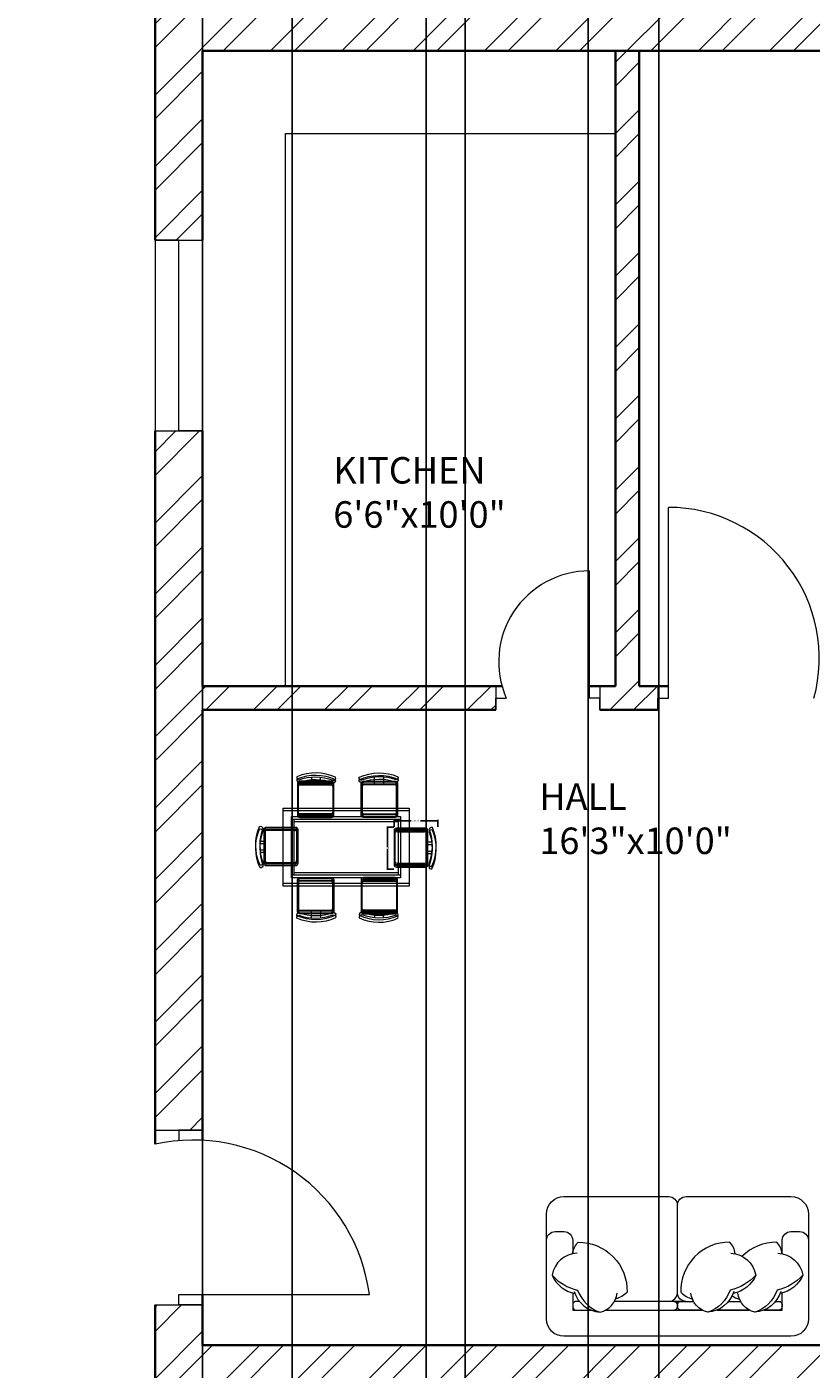
# Model space of a CAD drawing. Units: inches. Extents: x 2552 to 3217, y 1417 to 2737.
# Tile 5 of 25: x 2885 to 3033, y 1631 to 1885. Entities that reach past the tile are written whole.
import ezdxf

# ---------------------------------------------------------------- set-up
doc = ezdxf.new("R2010")
doc.units = ezdxf.units.IN
for name, color, linetype, lineweight in [('A-ANNO-DIMS', 2, 'Continuous', 18), ('A-AREA-IDEN', 7, 'Continuous', 18), ('A-DOOR', 21, 'Continuous', 18), ('A-FLOR-CASE', 9, 'Continuous', 18), ('A-FURN', 8, 'Continuous', 13), ('A-GLAZ', 161, 'Continuous', 18), ('A-WALL', 7, 'Continuous', 35), ('A-WALL-PATT', 217, 'Continuous', 13)]:
    doc.layers.add(name, color=color, linetype=linetype, lineweight=lineweight)
doc.styles.get("Standard").update_dxf_attribs({"font": 'arial.ttf'})
doc.dimstyles.get("Standard").update_dxf_attribs({"dimtxt": 0.18, "dimasz": 0.18, "dimexe": 0.18, "dimexo": 0.0625, "dimgap": 0.09, "dimtad": 0, "dimtih": 1, "dimtoh": 1, "dimdec": 4, "dimzin": 0, "dimdsep": 46, "dimtxsty": 'Standard', "dimcen": 0.09, "dimadec": 0, "dimazin": 0, "dimtfac": 1, "dimtdec": 4, "dimtofl": 0, "dimtmove": 0, "dimatfit": 3, "dimfxl": 1, "dimtolj": 1, "dimtzin": 0, "dimarcsym": 0})

# ---------------------------------------------------------------- blocks, each defined once
blk = doc.blocks.new('TABLE-DINING-RECT')
for points in [[(0, 14.74), (23.77, 14.74), (23.77, 0.48), (0, 0.48)], [(0, 14.74), (23.77, 14.74), (23.77, 0.48), (0, 0.48)], [(0, 14.26), (23.77, 14.26), (23.77, 0), (0, 0)], [(0, 14.26), (23.77, 14.26), (23.77, 0), (0, 0)], [(1.58, 13.15), (22.19, 13.15), (22.19, 2.06), (1.58, 2.06)], [(1.58, 13.15), (22.19, 13.15), (22.19, 2.06), (1.58, 2.06)], [(1.58, 12.68), (22.19, 12.68), (22.19, 1.59), (1.58, 1.59)], [(1.58, 12.68), (22.19, 12.68), (22.19, 1.58), (1.58, 1.58)], [(2.06, 12.68), (21.71, 12.68), (21.71, 2.54), (2.06, 2.54)], [(2.06, 12.68), (21.71, 12.68), (21.71, 2.54), (2.06, 2.54)], [(2.06, 12.2), (21.71, 12.2), (21.71, 2.06), (2.06, 2.06)], [(2.06, 12.2), (21.71, 12.2), (21.71, 2.06), (2.06, 2.06)]]:
    blk.add_lwpolyline(points, close=True)
blk = doc.blocks.new('DINING-CHAIR-EAST')
for points in [[(6.37, 7.27, 0.414214), (5.95, 7.69), (0.42, 7.69, 0.414214), (0, 7.27), (0, 1.26, 0.414214), (0.42, 0.84), (5.95, 0.84, 0.414214), (6.37, 1.26), (6.37, 7.27)], [(6.37, 7.27, 0.414214), (5.95, 7.69), (0.42, 7.69, 0.414214), (0, 7.27), (0, 1.26, 0.414214), (0.42, 0.84), (5.95, 0.84, 0.414214), (6.37, 1.26), (6.37, 7.27)], [(6.63, 7.46, -0.175809), (6.58, 0.99, 0.578392), (7.12, 0.5, 0.214524), (7.22, 7.8, 0.552014), (6.63, 7.46, -0.065079)], [(6.63, 7.46, -0.175809), (6.58, 0.99, 0.578392), (7.12, 0.49, 0.214524), (7.22, 7.8, 0.552014), (6.63, 7.46, -0.065079)], [(6.37, 6.8, 0.414214), (5.95, 7.22), (0.42, 7.22, 0.414214), (0, 6.8), (0, 0.78, 0.414214), (0.42, 0.36), (5.95, 0.36, 0.414214), (6.37, 0.78), (6.37, 6.8)], [(6.37, 6.8, 0.414214), (5.95, 7.22), (0.42, 7.22, 0.414214), (0, 6.8), (0, 0.78, 0.414214), (0.42, 0.36), (5.95, 0.36, 0.414214), (6.37, 0.78), (6.37, 6.8)], [(6.63, 6.98, -0.175809), (6.58, 0.51, 0.578392), (7.12, 0.02, 0.214524), (7.22, 7.33, 0.552014), (6.63, 6.98, -0.065079)], [(6.63, 6.98, -0.175809), (6.58, 0.51, 0.578392), (7.12, 0.02, 0.214524), (7.22, 7.33, 0.552014), (6.63, 6.98, -0.065079)], [(6.37, 3.37), (7.13, 3.37, -0.064759)], [(6.37, 3.37), (7.13, 3.37, -0.064759)], [(6.37, 2.9), (7.13, 2.9, -0.064759)], [(6.37, 2.9), (7.13, 2.9, -0.064759)]]:
    blk.add_lwpolyline(points, format="xyb")
for points in [[(6.18, 7.27), (6.18, 1.45, -0.414214), (5.76, 1.03), (0.61, 1.03, -0.414214), (0.19, 1.45), (0.19, 7.27, -0.512069), (0.61, 7.5), (5.76, 7.5, -0.512069)], [(6.18, 7.27), (6.18, 1.45, -0.414214), (5.76, 1.03), (0.61, 1.03, -0.414214), (0.19, 1.45), (0.19, 7.27, -0.512069), (0.61, 7.5), (5.76, 7.5, -0.512069)], [(6.18, 6.79), (6.18, 0.97, -0.414214), (5.76, 0.55), (0.61, 0.55, -0.414214), (0.19, 0.97), (0.19, 6.79, -0.512069), (0.61, 7.03), (5.76, 7.03, -0.512069)], [(6.18, 6.79), (6.18, 0.97, -0.414214), (5.76, 0.55), (0.61, 0.55, -0.414214), (0.19, 0.97), (0.19, 6.79, -0.512069), (0.61, 7.03), (5.76, 7.03, -0.512069)]]:
    blk.add_lwpolyline(points, format="xyb", close=True)
for points in [[(7.14, 5.05), (6.37, 5.05)], [(7.14, 5.05), (6.37, 5.05)], [(7.14, 4.58), (6.37, 4.58)], [(7.14, 4.58), (6.37, 4.58)]]:
    blk.add_lwpolyline(points)
blk = doc.blocks.new('WIN-36')
for p, q in [((4.5, 36), (0, 36)), ((0, 36), (9, 36)), ((0, 36), (0, 0)), ((4.5, 0), (4.5, 36)), ((9, 36), (9, 0)), ((0, 0), (9, 0)), ((9, 0), (4.5, 0))]:
    blk.add_line(p, q)
blk = doc.blocks.new('*D39')
at = {"layer": 'A-ANNO-DIMS', "color": 0, "lineweight": -2, "transparency": 16777216}
for p, q in [((2954.04, 1733.41), (2954.04, 1734.76)), ((2954.22, 1734.58), (2957.27, 1734.58)), ((2962.09, 1734.58), (2959.04, 1734.58)), ((2962.27, 1733.41), (2962.27, 1734.76))]:
    blk.add_line(p, q, dxfattribs=at)
at = {"layer": 'A-ANNO-DIMS', "color": 0, "transparency": 16777216}
for points in [[(2954.22, 1734.61), (2954.22, 1734.55), (2954.04, 1734.58)], [(2962.09, 1734.61), (2962.09, 1734.55), (2962.27, 1734.58)]]:
    blk.add_solid(points, dxfattribs=at)
at = {"layer": 'Defpoints', "color": 0, "transparency": 16777216}
for p in [(2962.27, 1734.58), (2954.04, 1733.35), (2962.27, 1733.35)]:
    blk.add_point(p, dxfattribs=at)
at = {"layer": 'A-ANNO-DIMS', "color": 0, "transparency": 16777216, "insert": (2958.16, 1734.58), "char_height": 0.18, "attachment_point": 5}
blk.add_mtext('\\A1;CHAIR 8 TYP.', dxfattribs=at)
blk = doc.blocks.new('*D40')
at = {"layer": 'A-ANNO-DIMS', "color": 0, "lineweight": -2, "transparency": 16777216}
for p, q in [((2953.98, 1733.35), (2952.63, 1733.35)), ((2952.81, 1733.17), (2952.81, 1729.58)), ((2952.81, 1725.63), (2952.81, 1729.22)), ((2953.98, 1725.45), (2952.63, 1725.45))]:
    blk.add_line(p, q, dxfattribs=at)
at = {"layer": 'A-ANNO-DIMS', "color": 0, "transparency": 16777216}
for points in [[(2952.78, 1733.17), (2952.84, 1733.17), (2952.81, 1733.35)], [(2952.78, 1725.63), (2952.84, 1725.63), (2952.81, 1725.45)]]:
    blk.add_solid(points, dxfattribs=at)
at = {"layer": 'Defpoints', "color": 0, "transparency": 16777216}
for p in [(2952.81, 1733.35), (2954.04, 1733.35), (2954.04, 1725.45)]:
    blk.add_point(p, dxfattribs=at)
at = {"layer": 'A-ANNO-DIMS', "color": 0, "transparency": 16777216, "insert": (2952.81, 1729.4), "char_height": 0.18, "attachment_point": 5}
blk.add_mtext('\\A1;8 TYP.', dxfattribs=at)
blk = doc.blocks.new('*D56')
at = {"layer": 'A-ANNO-DIMS', "color": 0, "lineweight": -2, "transparency": 16777216}
for p, q in [((2967.49, 2515.95), (2967.49, 1482.53)), ((2990.69, 2515.95), (2990.69, 1482.53)), ((2967.67, 1482.71), (2978.76, 1482.71)), ((2990.51, 1482.71), (2979.41, 1482.71))]:
    blk.add_line(p, q, dxfattribs=at)
at = {"layer": 'A-ANNO-DIMS', "color": 0, "transparency": 16777216}
for points in [[(2967.67, 1482.74), (2967.67, 1482.68), (2967.49, 1482.71)], [(2990.51, 1482.74), (2990.51, 1482.68), (2990.69, 1482.71)]]:
    blk.add_solid(points, dxfattribs=at)
at = {"layer": 'Defpoints', "color": 0, "transparency": 16777216}
for p in [(2967.49, 2516.01), (2990.69, 2516.01), (2990.69, 1482.71)]:
    blk.add_point(p, dxfattribs=at)
at = {"layer": 'A-ANNO-DIMS', "color": 0, "transparency": 16777216, "insert": (2979.09, 1482.71), "char_height": 0.18, "attachment_point": 5}
blk.add_mtext('\\A1;23.2', dxfattribs=at)
blk = doc.blocks.new('*D57')
at = {"layer": 'A-ANNO-DIMS', "color": 0, "lineweight": -2, "transparency": 16777216}
for p, q in [((3004.08, 2515.95), (3004.08, 1482.53)), ((3036.34, 2515.95), (3036.34, 1482.53)), ((3004.26, 1482.71), (3019.75, 1482.71)), ((3036.16, 1482.71), (3020.68, 1482.71))]:
    blk.add_line(p, q, dxfattribs=at)
at = {"layer": 'A-ANNO-DIMS', "color": 0, "transparency": 16777216}
for points in [[(3004.26, 1482.74), (3004.26, 1482.68), (3004.08, 1482.71)], [(3036.16, 1482.74), (3036.16, 1482.68), (3036.34, 1482.71)]]:
    blk.add_solid(points, dxfattribs=at)
at = {"layer": 'Defpoints', "color": 0, "transparency": 16777216}
for p in [(3004.08, 2516.01), (3036.34, 2516.01), (3036.34, 1482.71)]:
    blk.add_point(p, dxfattribs=at)
at = {"layer": 'A-ANNO-DIMS', "color": 0, "transparency": 16777216, "insert": (3020.21, 1482.71), "char_height": 0.18, "attachment_point": 5}
blk.add_mtext('\\A1;32.255', dxfattribs=at)
blk = doc.blocks.new('*D64')
at = {"layer": 'A-ANNO-DIMS', "color": 0, "lineweight": -2, "transparency": 16777216}
for p, q in [((2646.35, 1551.58), (2646.35, 2709.49)), ((2646.53, 2709.31), (2802.77, 2709.31)), ((2959.93, 2709.31), (2803.69, 2709.31)), ((2960.11, 1551.58), (2960.11, 2709.49))]:
    blk.add_line(p, q, dxfattribs=at)
at = {"layer": 'A-ANNO-DIMS', "color": 0, "transparency": 16777216}
for points in [[(2646.53, 2709.34), (2646.53, 2709.28), (2646.35, 2709.31)], [(2959.93, 2709.34), (2959.93, 2709.28), (2960.11, 2709.31)]]:
    blk.add_solid(points, dxfattribs=at)
at = {"layer": 'Defpoints', "color": 0, "transparency": 16777216}
for p in [(2960.11, 2709.31), (2646.35, 1551.51), (2960.11, 1551.51)]:
    blk.add_point(p, dxfattribs=at)
at = {"layer": 'A-ANNO-DIMS', "color": 0, "transparency": 16777216, "insert": (2803.23, 2709.31), "char_height": 0.18, "attachment_point": 5}
blk.add_mtext('\\A1;313.76', dxfattribs=at)
blk = doc.blocks.new('*D67')
at = {"layer": 'A-ANNO-DIMS', "color": 0, "lineweight": -2, "transparency": 16777216}
for p, q in [((2917.85, 2640.45), (2917.85, 1482.53)), ((2934.77, 2624.73), (2934.77, 1482.53)), ((2918.03, 1482.71), (2925.86, 1482.71)), ((2934.59, 1482.71), (2926.76, 1482.71))]:
    blk.add_line(p, q, dxfattribs=at)
at = {"layer": 'A-ANNO-DIMS', "color": 0, "transparency": 16777216}
for points in [[(2918.03, 1482.74), (2918.03, 1482.68), (2917.85, 1482.71)], [(2934.59, 1482.74), (2934.59, 1482.68), (2934.77, 1482.71)]]:
    blk.add_solid(points, dxfattribs=at)
at = {"layer": 'Defpoints', "color": 0, "transparency": 16777216}
for p in [(2917.85, 2640.51), (2934.77, 2624.79), (2934.77, 1482.71)]:
    blk.add_point(p, dxfattribs=at)
at = {"layer": 'A-ANNO-DIMS', "color": 0, "transparency": 16777216, "insert": (2926.31, 1482.71), "char_height": 0.18, "attachment_point": 5}
blk.add_mtext('\\A1;16.912', dxfattribs=at)

msp = doc.modelspace()

# ---------------------------------------------------------------- hatches: boundary and pattern name
at = {"layer": 'A-WALL-PATT'}
h = msp.add_hatch(dxfattribs=at)
h.set_pattern_fill('ANSI32', color=256)
h.paths.add_polyline_path([(2756.676, 2649.5125), (2637.3535, 2649.5125), (2637.3535, 2617.9626), (2641.8535, 2617.9626), (2646.3535, 2617.9626), (2646.3535, 2640.5125), (2724.3535, 2640.5125), (2724.3535, 2520.5125), (2720.299, 2520.5125), (2720.299, 2516.0125), (2733.4075, 2516.0125), (2733.4075, 2518.2213), (2733.4075, 2520.5125), (2728.8535, 2520.5125), (2728.8535, 2640.5125), (2756.676, 2640.5125)])
h.paths.add_polyline_path([(2848.8535, 2649.5125), (2804.676, 2649.5125), (2804.676, 2640.5125), (2839.8535, 2640.5125), (2839.8535, 2598.3517), (2848.8535, 2598.3517)])
h.paths.add_polyline_path([(2646.3535, 2516.0125), (2697.9593, 2516.0125), (2697.9593, 2518.2625), (2697.9593, 2520.5125), (2646.3535, 2520.5125), (2646.3535, 2581.9626), (2637.3535, 2581.9626), (2637.3535, 2364.3298), (2646.3535, 2364.3298), (2646.3535, 2387.0125), (2724.3535, 2387.0125), (2724.3535, 2267.0125), (2721.0443, 2267.0125), (2721.0443, 2262.5125), (2733.7854, 2262.5125), (2733.7854, 2264.7625), (2733.7854, 2267.0125), (2728.8535, 2267.0125), (2728.8535, 2387.0125), (2839.8535, 2387.0125), (2839.8535, 2363.8387), (2848.8535, 2363.8387), (2848.8535, 2403.7415), (2844.3535, 2403.7415), (2839.8535, 2403.7415), (2839.8535, 2396.0125), (2646.3535, 2396.0125)])
h.paths.add_polyline_path([(2848.8535, 2550.3517), (2844.3535, 2550.3517), (2839.8535, 2550.3517), (2839.8535, 2520.5125), (2801.9195, 2520.5125), (2801.9195, 2518.2625), (2801.9195, 2516.0125), (2839.8535, 2516.0125), (2839.8535, 2507.5813), (2848.8535, 2507.5813)], flags=17)
h.paths.add_polyline_path([(2848.8535, 2483.5813), (2844.3535, 2483.5813), (2839.8535, 2483.5813), (2839.8535, 2468.0125), (2773.8535, 2468.0125), (2773.8535, 2516.0125), (2778.1336, 2516.0125), (2778.1336, 2520.5125), (2766.696, 2520.5125), (2766.696, 2518.2625), (2766.696, 2516.0125), (2769.3535, 2516.0125), (2769.3535, 2463.5125), (2839.8535, 2463.5125), (2839.8535, 2431.0782), (2848.8535, 2431.0782)], flags=17)
h.paths.add_polyline_path([(2917.8535, 2569.2764), (2913.3535, 2569.2764), (2908.8535, 2569.2764), (2908.8535, 2433.001), (2917.8535, 2433.001), (2917.8535, 2516.0125), (2967.486, 2516.0125), (2967.486, 2520.5125), (2917.8535, 2520.5125)])
h.paths.add_polyline_path([(3000.3535, 2640.5125), (2995.8535, 2640.5125), (2995.8535, 2520.5125), (2990.688, 2520.5125), (2990.688, 2516.0125), (3004.0844, 2516.0125), (3004.0844, 2518.2625), (3004.0844, 2520.5125), (3000.3535, 2520.5125)])
h.paths.add_polyline_path([(3120.3535, 2561.3689), (3115.8535, 2561.3689), (3111.3535, 2561.3689), (3111.3535, 2520.5125), (3070.9814, 2520.5125), (3070.9814, 2518.2625), (3070.9814, 2516.0125), (3111.3535, 2516.0125), (3111.3535, 2505.1841), (3120.3535, 2505.1841)])
h.paths.add_polyline_path([(3120.3535, 2481.1841), (3115.8535, 2481.1841), (3111.3535, 2481.1841), (3111.3535, 2468.0125), (3045.3535, 2468.0125), (3045.3535, 2516.0125), (3048.9787, 2516.0125), (3048.9787, 2520.5125), (3036.3395, 2520.5125), (3036.3395, 2516.0125), (3040.8535, 2516.0125), (3040.8535, 2463.5125), (3111.3535, 2463.5125), (3111.3535, 2396.0125), (2917.8535, 2396.0125), (2917.8535, 2403.4124), (2913.3535, 2403.4124), (2908.8535, 2403.4124), (2908.8535, 2182.5756), (2917.8535, 2182.5756), (2917.8535, 2262.5125), (2968.001, 2262.5125), (2968.001, 2264.7625), (2968.001, 2267.0125), (2917.8535, 2267.0125), (2917.8535, 2387.0125), (3111.3535, 2387.0125), (3111.3535, 2352.2435), (3120.3535, 2352.2435)])
h.paths.add_polyline_path([(3120.3535, 2304.2435), (3115.8535, 2304.2435), (3111.3535, 2304.2435), (3111.3535, 2267.0125), (3073.8616, 2267.0125), (3073.8616, 2264.7625), (3073.8616, 2262.5125), (3111.3535, 2262.5125), (3111.3535, 2252.376), (3120.3535, 2252.376)], flags=17)
h.paths.add_polyline_path([(3120.3535, 2228.376), (3115.8535, 2228.376), (3111.3535, 2228.376), (3111.3535, 2214.5125), (3045.3535, 2214.5125), (3045.3535, 2262.5125), (3049.3096, 2262.5125), (3049.3096, 2267.0125), (3035.0125, 2267.0125), (3035.0125, 2262.5125), (3040.8535, 2262.5125), (3040.8535, 2210.0125), (3111.3535, 2210.0125), (3111.3535, 2142.5125), (2917.8535, 2142.5125), (2917.8535, 2150.2408), (2913.3535, 2150.2408), (2908.8535, 2150.2408), (2908.8535, 1924.9905), (2917.8535, 1924.9905), (2917.8535, 2009.0125), (2971.959, 2009.0125), (2971.959, 2011.2625), (2971.959, 2013.5125), (2917.8535, 2013.5125), (2917.8535, 2133.5125), (2995.8535, 2133.5125), (2995.8535, 2013.5125), (2992.1797, 2013.5125), (2992.1797, 2009.0125), (3004.3344, 2009.0125), (3004.3344, 2011.2625), (3004.3344, 2013.5125), (3000.3535, 2013.5125), (3000.3535, 2133.5125), (3111.3535, 2133.5125), (3111.3535, 2115.0291), (3120.3535, 2115.0291)])
h.paths.add_polyline_path([(3000.3535, 2387.0125), (2995.8535, 2387.0125), (2995.8535, 2267.0125), (2991.3326, 2267.0125), (2991.3326, 2262.5125), (3004.1044, 2262.5125), (3004.1044, 2264.7625), (3004.1044, 2267.0125), (3000.3535, 2267.0125)], flags=17)
h.paths.add_polyline_path([(3120.3535, 1973.2388), (3115.8535, 1973.2388), (3111.3535, 1973.2388), (3111.3535, 1961.0125), (3045.3535, 1961.0125), (3045.3535, 2009.0125), (3048.9101, 2009.0125), (3048.9101, 2013.5125), (3037.105, 2013.5125), (3037.105, 2011.2625), (3037.105, 2009.0125), (3040.8535, 2009.0125), (3040.8535, 1956.5125), (3111.3535, 1956.5125), (3111.3535, 1889.0125), (2917.8535, 1889.0125), (2917.8535, 1895.7215), (2913.3535, 1895.7215), (2908.8535, 1895.7215), (2908.8535, 1844.2217), (2917.8535, 1844.2217), (2917.8535, 1880.0125), (3111.3535, 1880.0125), (3111.3535, 1846.9541), (3120.3535, 1846.9541)])
h.paths.add_polyline_path([(3120.3535, 2067.0291), (3111.3535, 2067.0291), (3111.3535, 2013.5125), (3071.3001, 2013.5125), (3071.3001, 2009.0125), (3111.3535, 2009.0125), (3111.3535, 1997.2388), (3120.3535, 1997.2388)], flags=0)
h.paths.add_polyline_path([(3120.3535, 1798.9541), (3115.8535, 1798.9541), (3111.3535, 1798.9541), (3111.3535, 1760.0125), (3071.2497, 1760.0125), (3071.2497, 1757.7625), (3071.2497, 1755.5125), (3111.3535, 1755.5125), (3111.3535, 1746.162), (3120.3535, 1746.2478)])
h.paths.add_polyline_path([(3120.3535, 1722.2049), (3111.3535, 1722.2049), (3111.3535, 1707.5125), (3045.3535, 1707.5125), (3045.3535, 1755.5125), (3048.6624, 1755.5125), (3048.6624, 1760.0125), (3035.3703, 1760.0125), (3035.3703, 1755.5125), (3040.8535, 1755.5125), (3040.8535, 1703.0125), (3111.3535, 1703.0125), (3111.3535, 1635.5125), (2917.8535, 1635.5125), (2917.8535, 1643.1366), (2913.3535, 1643.1366), (2908.8535, 1643.1366), (2908.8535, 1626.5125), (3120.3535, 1626.5125)])
h.paths.add_polyline_path([(2917.8535, 1755.5125), (2973.2287, 1755.5125), (2973.2287, 1757.7625), (2973.2287, 1760.0125), (2917.8535, 1760.0125), (2917.8535, 1808.2217), (2913.3535, 1808.2217), (2908.8535, 1808.2217), (2908.8535, 1676.1665), (2917.8535, 1676.1665)])
h.paths.add_polyline_path([(3000.3535, 1880.0125), (2995.8535, 1880.0125), (2995.8535, 1760.0125), (2992.9329, 1760.0125), (2992.9329, 1755.5125), (3003.8766, 1755.5125), (3003.8766, 1757.7625), (3003.8766, 1760.0125), (3000.3535, 1760.0125)])
h.paths.add_polyline_path([(2848.8535, 1896.6971), (2844.3535, 1896.6971), (2839.8535, 1896.6971), (2839.8535, 1889.0125), (2646.3535, 1889.0125), (2646.3535, 2009.0125), (2700.5253, 2009.0125), (2700.5253, 2011.2625), (2700.5253, 2013.5125), (2646.3535, 2013.5125), (2646.3535, 2053.1812), (2641.8535, 2053.1812), (2637.3535, 2053.1812), (2637.3535, 1836.254), (2646.3535, 1836.254), (2646.3535, 1880.0125), (2724.3535, 1880.0125), (2724.3535, 1760.0125), (2721.2473, 1760.0125), (2721.2473, 1755.5125), (2731.9187, 1755.5125), (2731.9187, 1757.7625), (2731.9187, 1760.0125), (2728.8535, 1760.0125), (2728.8535, 1880.0125), (2839.8535, 1880.0125), (2839.8535, 1840.3813), (2848.8535, 1840.3813)])
h.paths.add_polyline_path([(2848.8535, 1792.3813), (2844.3535, 1792.3813), (2839.8535, 1792.3813), (2839.8535, 1760.0125), (2797.8845, 1760.0125), (2797.8845, 1755.5125), (2839.8535, 1755.5125), (2839.8535, 1743.3688), (2844.3535, 1743.3688), (2848.8535, 1743.3688)], flags=0)
h.paths.add_polyline_path([(2848.8535, 1719.3688), (2844.3535, 1719.3688), (2839.8535, 1719.3688), (2839.8535, 1707.5125), (2773.8535, 1707.5125), (2773.8535, 1755.5125), (2777.716, 1755.5125), (2777.716, 1760.0125), (2760.9247, 1760.0125), (2760.9247, 1757.9721), (2760.9247, 1755.5125), (2769.3535, 1755.5125), (2769.3535, 1703.0125), (2839.8535, 1703.0125), (2839.8535, 1673.0277), (2848.8535, 1672.9407)], flags=0)
h.paths.add_polyline_path([(2646.3535, 1755.5125), (2702.9171, 1755.5125), (2702.9171, 1757.7625), (2702.9171, 1760.0125), (2646.3535, 1760.0125), (2646.3535, 1800.254), (2641.8535, 1800.254), (2637.3535, 1800.254), (2637.3535, 1626.5125), (2848.8535, 1626.5125), (2848.8535, 1643.1187), (2844.3535, 1643.1187), (2839.8535, 1643.1187), (2839.8535, 1635.5125), (2646.3535, 1635.5125)])
h.paths.add_polyline_path([(2848.8535, 2148.8427), (2844.3535, 2148.8427), (2839.8535, 2148.8427), (2839.8535, 2142.5125), (2646.3535, 2142.5125), (2646.3535, 2262.5125), (2701.3562, 2262.5125), (2701.3562, 2264.7625), (2701.3562, 2267.0125), (2646.3535, 2267.0125), (2646.3535, 2328.3298), (2637.3535, 2328.3298), (2637.3535, 2089.1812), (2646.3535, 2089.1812), (2646.3535, 2133.5125), (2839.8535, 2133.5125), (2839.8535, 2097.5966), (2848.8535, 2097.5966)])
h.paths.add_polyline_path([(2728.8535, 2133.5125), (2724.3535, 2133.5125), (2724.3535, 2013.5125), (2719.6039, 2013.5125), (2719.6039, 2009.0125), (2732.5784, 2009.0125), (2732.5784, 2011.2625), (2732.5784, 2013.5125), (2728.8535, 2013.5125)])
h.paths.add_polyline_path([(2848.8535, 1970.0557), (2844.3535, 1970.0557), (2839.8535, 1970.0557), (2839.8535, 1961.0125), (2773.8535, 1961.0125), (2773.8535, 2009.0125), (2777.3388, 2009.0125), (2777.3388, 2013.5125), (2764.7681, 2013.5125), (2764.7681, 2009.0125), (2769.3535, 2009.0125), (2769.3535, 1956.5125), (2839.8535, 1956.5125), (2839.8535, 1924.7199), (2848.8535, 1924.7199)], flags=17)
h.paths.add_polyline_path([(2848.8535, 2049.5966), (2844.3535, 2049.5966), (2839.8535, 2049.5966), (2839.8535, 2013.5125), (2798.198, 2013.5125), (2798.198, 2011.2625), (2798.198, 2009.0125), (2839.8535, 2009.0125), (2839.8535, 1994.0557), (2848.8535, 1994.0557)], flags=17)
h.paths.add_polyline_path([(2848.8535, 2315.8387), (2839.8535, 2315.8387), (2839.8535, 2267.0125), (2799.3375, 2267.0125), (2799.3375, 2264.7625), (2799.3375, 2262.5125), (2839.8535, 2262.5125), (2839.8535, 2253.2843), (2848.8535, 2253.2843)], flags=17)
h.paths.add_polyline_path([(2848.8535, 2229.2843), (2839.8535, 2229.2843), (2839.8535, 2177.6936), (2848.8535, 2177.6936)], flags=17)
h.paths.add_polyline_path([(2839.8535, 2214.5125), (2773.8535, 2214.5125), (2773.8535, 2262.5125), (2777.6984, 2262.5125), (2777.6984, 2267.0125), (2763.8226, 2267.0125), (2763.8226, 2262.5125), (2769.3535, 2262.5125), (2769.3535, 2210.0125), (2839.8535, 2210.0125)], flags=17)
h.paths.add_polyline_path([(3050.32, 2520.2817), (3088.9114, 2520.2817), (3088.9114, 2538.939), (3050.32, 2538.939)], flags=9)

# ---------------------------------------------------------------- linework, layer by layer
at = {"layer": 'A-DOOR'}
for p, q in [((3005.8766, 1757.7625), (3005.8766, 1793.7625)), ((2990.9329, 1757.7625), (2990.9329, 1781.7625)), ((2973.2287, 1760.0125), (2973.2287, 1755.5125)), ((2992.9329, 1760.0125), (2992.9329, 1755.5125)), ((3003.8766, 1760.0125), (3003.8766, 1755.5125)), ((2973.2287, 1755.5125), (2973.2287, 1757.7625)), ((2973.2287, 1757.7625), (2975.2287, 1757.7625)), ((2992.9329, 1757.7625), (2990.9329, 1757.7625)), ((2992.9329, 1755.5125), (2992.9329, 1757.7625)), ((3003.8766, 1755.5125), (3003.8766, 1757.7625)), ((3003.8766, 1757.7625), (3005.8766, 1757.7625)), ((2908.8535, 1676.1665), (2917.8535, 1676.1665)), ((2917.8535, 1676.1665), (2913.3535, 1676.1665)), ((2913.3535, 1676.1665), (2913.3535, 1674.1665)), ((2908.8535, 1643.1366), (2917.8535, 1643.1366)), ((2913.3535, 1643.1366), (2913.3535, 1645.1366)), ((2913.3535, 1645.1366), (2949.3535, 1645.1366)), ((2917.8535, 1643.1366), (2913.3535, 1643.1366)), ((2913.3535, 1643.1366), (2913.3535, 1643.1366))]:
    msp.add_line(p, q, dxfattribs=at)
for centre, radius, start, end in [((3005.8766, 1765.2638), 28.4987, 344.739016, 90), ((2990.9329, 1764.6246), 17.1379, 90, 203.603435), ((2916.0572, 1640.6826), 33.5929, 7.619186, 102.382716)]:
    msp.add_arc(centre, radius, start, end, dxfattribs=at)
at = {"layer": 'A-FLOR-CASE'}
for p, q in [((2933.5182, 1760.0125), (2933.5182, 1864.3833)), ((2933.5182, 1864.3833), (2995.8535, 1864.3833))]:
    msp.add_line(p, q, dxfattribs=at)
at = {"layer": 'A-FURN'}
for points in [[(2936.0194, 1742.3042, -0.17580919), (2942.4939, 1742.2552, 0.57839206), (2942.9843, 1742.7945, 0.21452438), (2935.6761, 1742.8926, 0.55201397), (2936.0194, 1742.3042, -0.06507904)], [(2936.0194, 1742.304, -0.17580919), (2942.4939, 1742.2549, 0.57839206), (2942.9844, 1742.7943, 0.21452438), (2935.6761, 1742.8923, 0.55201397), (2936.0194, 1742.304, -0.06507904)], [(2936.0194, 1741.8288, -0.17580919), (2942.4939, 1741.7798, 0.57839206), (2942.9843, 1742.3191, 0.21452438), (2935.6761, 1742.4172, 0.55201397), (2936.0194, 1741.8288, -0.06507904)], [(2936.0194, 1741.8286, -0.17580919), (2942.4939, 1741.7795, 0.57839206), (2942.9844, 1742.3189, 0.21452438), (2935.6761, 1742.4169, 0.55201397), (2936.0194, 1741.8286, -0.06507904)], [(2942.2192, 1742.0444), (2936.2085, 1742.0444, 0.41421356), (2935.788, 1741.6238), (2935.788, 1736.0972, 0.41421356), (2936.2085, 1735.6766), (2942.2192, 1735.6766, 0.41421356), (2942.6397, 1736.0972), (2942.6397, 1741.6238, 0.41421356), (2942.2192, 1742.0444)], [(2942.2192, 1742.0441), (2936.2085, 1742.0441, 0.41421356), (2935.788, 1741.6236), (2935.788, 1736.0969, 0.41421356), (2936.2085, 1735.6764), (2942.2192, 1735.6764, 0.41421356), (2942.6397, 1736.0969), (2942.6397, 1741.6236, 0.41421356), (2942.2192, 1742.0441)], [(2942.2192, 1741.5689), (2936.2085, 1741.5689, 0.41421356), (2935.788, 1741.1484), (2935.788, 1735.6217, 0.41421356), (2936.2085, 1735.2012), (2942.2192, 1735.2012, 0.41421356), (2942.6397, 1735.6217), (2942.6397, 1741.1484, 0.41421356), (2942.2192, 1741.5689)], [(2942.2192, 1741.5687), (2936.2085, 1741.5687, 0.41421356), (2935.788, 1741.1482), (2935.788, 1735.6215, 0.41421356), (2936.2085, 1735.201), (2942.2192, 1735.201, 0.41421356), (2942.6397, 1735.6215), (2942.6397, 1741.1482, 0.41421356), (2942.2192, 1741.5687)], [(2940.1079, 1742.0444), (2940.1079, 1742.8045, -0.06475861)], [(2940.1079, 1742.0441), (2940.1079, 1742.8043, -0.06475861)], [(2940.1079, 1741.5689), (2940.1079, 1742.3291, -0.06475861)], [(2940.1079, 1741.5687), (2940.1079, 1742.3289, -0.06475861)], [(2947.9445, 1742.2552, -0.57839206), (2947.454, 1742.7945, -0.21452438), (2954.7623, 1742.8926, -0.55201397), (2954.419, 1742.3042, 0.1758092), (2947.9445, 1742.2552)], [(2947.9445, 1742.2549, -0.57839206), (2947.454, 1742.7943, -0.21452438), (2954.7623, 1742.8923, -0.55201397), (2954.419, 1742.304, 0.1758092), (2947.9445, 1742.2549)], [(2947.9445, 1741.7798, -0.57839206), (2947.454, 1742.3191, -0.21452438), (2954.7623, 1742.4172, -0.55201397), (2954.419, 1741.8288, 0.1758092), (2947.9445, 1741.7798)], [(2947.9445, 1741.7795, -0.57839206), (2947.454, 1742.3189, -0.21452438), (2954.7623, 1742.4169, -0.55201397), (2954.419, 1741.8286, 0.1758092), (2947.9445, 1741.7795)], [(2954.2299, 1742.0444, -0.41421356), (2954.6504, 1741.6238), (2954.6504, 1736.0972, -0.41421356), (2954.2299, 1735.6766), (2948.2192, 1735.6766, -0.41421356), (2947.7987, 1736.0972), (2947.7987, 1741.6238, -0.41421356), (2948.2192, 1742.0444), (2954.2299, 1742.0444)], [(2954.2299, 1742.0441, -0.41421356), (2954.6504, 1741.6236), (2954.6504, 1736.0969, -0.41421356), (2954.2299, 1735.6764), (2948.2192, 1735.6764, -0.41421356), (2947.7987, 1736.0969), (2947.7987, 1741.6236, -0.41421356), (2948.2192, 1742.0441), (2954.2299, 1742.0441)], [(2954.2299, 1741.5689, -0.41421356), (2954.6504, 1741.1484), (2954.6504, 1735.6217, -0.41421356), (2954.2299, 1735.2012), (2948.2192, 1735.2012, -0.41421356), (2947.7987, 1735.6217), (2947.7987, 1741.1484, -0.41421356), (2948.2192, 1741.5689), (2954.2299, 1741.5689)], [(2954.2299, 1741.5687, -0.41421356), (2954.6504, 1741.1482), (2954.6504, 1735.6215, -0.41421356), (2954.2299, 1735.201), (2948.2192, 1735.201, -0.41421356), (2947.7987, 1735.6215), (2947.7987, 1741.1482, -0.41421356), (2948.2192, 1741.5687), (2954.2299, 1741.5687)], [(2950.3304, 1742.0444), (2950.3304, 1742.8045, 0.06475861)], [(2950.3304, 1741.5689), (2950.3304, 1742.3291, 0.06475861)], [(2950.3305, 1742.0441), (2950.3305, 1742.8043, 0.06475861)], [(2950.3305, 1741.5687), (2950.3305, 1742.3289, 0.06475861)], [(2929.2459, 1726.6694, -0.57839206), (2928.7066, 1726.1789, -0.21452438), (2928.6085, 1733.4872, -0.55201397), (2929.1969, 1733.1438, 0.17580937), (2929.2459, 1726.6694)], [(2929.2459, 1726.6691, -0.57839206), (2928.7066, 1726.1787, -0.21452438), (2928.6085, 1733.4869, -0.55201397), (2929.1969, 1733.1436, 0.17580937), (2929.2459, 1726.6691)], [(2929.2459, 1726.194, -0.57839206), (2928.7066, 1725.7035, -0.21452438), (2928.6085, 1733.0118, -0.55201397), (2929.1969, 1732.6684, 0.17580937), (2929.2459, 1726.194)], [(2929.2459, 1726.1937, -0.57839206), (2928.7066, 1725.7032, -0.21452438), (2928.6085, 1733.0115, -0.55201397), (2929.1969, 1732.6682, 0.17580937), (2929.2459, 1726.1937)], [(2929.4567, 1732.9547, -0.41421356), (2929.8772, 1733.3753), (2935.4039, 1733.3753, -0.41421356), (2935.8244, 1732.9547), (2935.8244, 1726.9441, -0.41421356), (2935.4039, 1726.5236), (2929.8772, 1726.5236, -0.41421356), (2929.4567, 1726.9441), (2929.4567, 1732.9547)], [(2929.4567, 1732.9545, -0.41421356), (2929.8772, 1733.375), (2935.4039, 1733.375, -0.41421356), (2935.8244, 1732.9545), (2935.8244, 1726.9438, -0.41421356), (2935.4039, 1726.5233), (2929.8772, 1726.5233, -0.41421356), (2929.4567, 1726.9438), (2929.4567, 1732.9545)], [(2929.4567, 1732.4793, -0.41421356), (2929.8772, 1732.8998), (2935.4039, 1732.8998, -0.41421356), (2935.8244, 1732.4793), (2935.8244, 1726.4687, -0.41421356), (2935.4039, 1726.0482), (2929.8772, 1726.0482, -0.41421356), (2929.4567, 1726.4687), (2929.4567, 1732.4793)], [(2929.4567, 1732.4791, -0.41421356), (2929.8772, 1732.8996), (2935.4039, 1732.8996, -0.41421356), (2935.8244, 1732.4791), (2935.8244, 1726.4684, -0.41421356), (2935.4039, 1726.0479), (2929.8772, 1726.0479, -0.41421356), (2929.4567, 1726.4684), (2929.4567, 1732.4791)], [(2929.4567, 1729.0553), (2928.6966, 1729.0553, 0.06475861)], [(2929.4567, 1729.0551), (2928.6966, 1729.0551, 0.06475861)], [(2929.4567, 1728.5799), (2928.6966, 1728.5799, 0.06475861)], [(2929.4567, 1728.5797), (2928.6966, 1728.5797, 0.06475861)], [(2942.2192, 1717.4769), (2936.2085, 1717.4769, -0.41421356), (2935.788, 1717.8974), (2935.788, 1723.4241, -0.41421356), (2936.2085, 1723.8446), (2942.2192, 1723.8446, -0.41421356), (2942.6397, 1723.4241), (2942.6397, 1717.8974, -0.41421356), (2942.2192, 1717.4769)], [(2942.2192, 1717.4766), (2936.2085, 1717.4766, -0.41421356), (2935.788, 1717.8971), (2935.788, 1723.4238, -0.41421356), (2936.2085, 1723.8443), (2942.2192, 1723.8443, -0.41421356), (2942.6397, 1723.4238), (2942.6397, 1717.8971, -0.41421356), (2942.2192, 1717.4766)], [(2954.2299, 1717.4769, 0.41421356), (2954.6504, 1717.8974), (2954.6504, 1723.4241, 0.41421356), (2954.2299, 1723.8446), (2948.2192, 1723.8446, 0.41421356), (2947.7987, 1723.4241), (2947.7987, 1717.8974, 0.41421356), (2948.2192, 1717.4769), (2954.2299, 1717.4769)], [(2954.2299, 1717.4766, 0.41421356), (2954.6504, 1717.8971), (2954.6504, 1723.4238, 0.41421356), (2954.2299, 1723.8443), (2948.2192, 1723.8443, 0.41421356), (2947.7987, 1723.4238), (2947.7987, 1717.8971, 0.41421356), (2948.2192, 1717.4766), (2954.2299, 1717.4766)], [(2942.2192, 1717.0015), (2936.2085, 1717.0015, -0.41421356), (2935.788, 1717.422), (2935.788, 1722.9487, -0.41421356), (2936.2085, 1723.3692), (2942.2192, 1723.3692, -0.41421356), (2942.6397, 1722.9487), (2942.6397, 1717.422, -0.41421356), (2942.2192, 1717.0015)], [(2942.2192, 1717.0012), (2936.2085, 1717.0012, -0.41421356), (2935.788, 1717.4217), (2935.788, 1722.9484, -0.41421356), (2936.2085, 1723.3689), (2942.2192, 1723.3689, -0.41421356), (2942.6397, 1722.9484), (2942.6397, 1717.4217, -0.41421356), (2942.2192, 1717.0012)], [(2954.2299, 1717.0015, 0.41421356), (2954.6504, 1717.422), (2954.6504, 1722.9487, 0.41421356), (2954.2299, 1723.3692), (2948.2192, 1723.3692, 0.41421356), (2947.7987, 1722.9487), (2947.7987, 1717.422, 0.41421356), (2948.2192, 1717.0015), (2954.2299, 1717.0015)], [(2954.2299, 1717.0012, 0.41421356), (2954.6504, 1717.4217), (2954.6504, 1722.9484, 0.41421356), (2954.2299, 1723.3689), (2948.2192, 1723.3689, 0.41421356), (2947.7987, 1722.9484), (2947.7987, 1717.4217, 0.41421356), (2948.2192, 1717.0012), (2954.2299, 1717.0012)], [(2942.4939, 1717.2661, -0.57839206), (2942.9843, 1716.7267, -0.21452438), (2935.6761, 1716.6287, -0.55201397), (2936.0194, 1717.217, 0.17580929), (2942.4939, 1717.2661)], [(2942.4939, 1717.2658, -0.57839206), (2942.9844, 1716.7265, -0.21452438), (2935.6761, 1716.6284, -0.55201397), (2936.0194, 1717.2168, 0.17580929), (2942.4939, 1717.2658)], [(2942.4939, 1716.7906, -0.57839206), (2942.9843, 1716.2513, -0.21452438), (2935.6761, 1716.1533, -0.55201397), (2936.0194, 1716.7416, 0.17580929), (2942.4939, 1716.7906)], [(2942.4939, 1716.7904, -0.57839206), (2942.9844, 1716.2511, -0.21452438), (2935.6761, 1716.153, -0.55201397), (2936.0194, 1716.7414, 0.17580929), (2942.4939, 1716.7904)], [(2940.1079, 1717.4769), (2940.1079, 1716.7167, 0.06475861)], [(2940.1079, 1717.4766), (2940.1079, 1716.7165, 0.06475861)], [(2940.1079, 1717.0015), (2940.1079, 1716.2413, 0.06475861)], [(2940.1079, 1717.0012), (2940.1079, 1716.2411, 0.06475861)], [(2954.419, 1717.217, -0.17580928), (2947.9445, 1717.2661, 0.57839206), (2947.454, 1716.7267, 0.21452438), (2954.7623, 1716.6287, 0.55201397), (2954.419, 1717.217, -0.06507904)], [(2954.419, 1717.2168, -0.17580928), (2947.9445, 1717.2658, 0.57839206), (2947.454, 1716.7265, 0.21452438), (2954.7623, 1716.6284, 0.55201397), (2954.419, 1717.2168, -0.06507904)], [(2954.419, 1716.7416, -0.17580928), (2947.9445, 1716.7906, 0.57839206), (2947.454, 1716.2513, 0.21452438), (2954.7623, 1716.1533, 0.55201397), (2954.419, 1716.7416, -0.06507904)], [(2954.419, 1716.7414, -0.17580928), (2947.9445, 1716.7904, 0.57839206), (2947.454, 1716.2511, 0.21452438), (2954.7623, 1716.153, 0.55201397), (2954.419, 1716.7414, -0.06507904)], [(2950.3304, 1717.4769), (2950.3304, 1716.7167, -0.06475861)], [(2950.3304, 1717.0015), (2950.3304, 1716.2413, -0.06475861)], [(2950.3305, 1717.4766), (2950.3305, 1716.7165, -0.06475861)], [(2950.3305, 1717.0012), (2950.3305, 1716.2411, -0.06475861)], [(3005.9224, 1643.8104, 0.41421356), (3007.572, 1645.46), (3007.572, 1661.9556, 0.41421356)], [(3009.2215, 1643.8104, -0.41421356), (3007.572, 1645.46), (3007.572, 1661.9556, -0.41421356)], [(2982.8285, 1655.3574, -0.41421356), (2984.4781, 1657.0069), (2986.1277, 1657.0069, -0.41421356), (2987.7772, 1655.3574), (2987.7772, 1652.8016)], [(3027.3667, 1652.8016), (3027.3667, 1655.3574, -0.41421356), (3029.0163, 1657.0069), (3030.6659, 1657.0069, -0.41421356), (3032.3154, 1655.3574)], [(2988.605, 1652.9014, 0.35677236), (2983.8784, 1648.7435, 0.24954205), (2988.1612, 1645.317, -9.61688035)], [(2987.7736, 1652.8008, -0.16554063), (2988.7941, 1654.9804, -0.42598917), (2998.0584, 1645.5306, -0.12152332), (2995.8592, 1644.2281, 7.11546429)], [(3018.4842, 1652.8008, 0.16554063), (3017.4637, 1654.9804, 0.42598917), (3008.1995, 1645.5306, 0.12152332), (3010.3986, 1644.2281, -7.11546429)], [(3017.6528, 1652.9014, -0.35677236), (3022.3795, 1648.7435, -0.24954205), (3018.0967, 1645.317, 9.61688035)], [(3027.3703, 1652.8008, 0.16554063), (3026.3499, 1654.9804, 0.20023115), (3019.8017, 1652.3259, 0.12152332)], [(3026.5389, 1652.9014, -0.35677236), (3031.2656, 1648.7435, -0.24954205), (3026.9828, 1645.317, 9.61688035)], [(2983.8784, 1648.7435, 0.14772988), (2988.6996, 1645.9086, 0.21334276), (2992.9536, 1641.7507, 0.17866181)], [(3022.3795, 1648.7435, -0.14772988), (3017.5583, 1645.9086, -0.21334276), (3013.3043, 1641.7507, -0.17866181)], [(3031.2656, 1648.7435, -0.14772988), (3026.4444, 1645.9086, -0.21334276), (3022.1904, 1641.7507, -0.17866181)], [(2988.0335, 1645.6826, 0.30666349), (2992.9536, 1641.7507, 0.30632997), (2996.1677, 1645.3416, -0.87284716)], [(3005.9224, 1643.8104, 0.41421356), (3007.572, 1645.46)], [(3009.2215, 1643.8104, -0.41421356), (3007.572, 1645.46)], [(3018.2243, 1645.6826, -0.30666349), (3013.3043, 1641.7507, -0.30632997), (3010.0901, 1645.3416, 0.87284716)], [(3027.1104, 1645.6826, -0.30666349), (3022.1904, 1641.7507, -0.30632997), (3018.9763, 1645.3416, 0.87284716)], [(3023.8965, 1642.1609), (3027.3667, 1642.1609), (3027.3667, 1645.4026, -0.41421356)], [(2989.036, 1643.8104), (2988.437, 1643.8104, 0.41421356), (2987.7772, 1643.1506), (2987.7772, 1642.8207, 0.41421356), (2988.437, 1642.1609)], [(2993.9917, 1642.1609), (3006.9122, 1642.1609, 0.41421356), (3007.572, 1642.8207), (3007.572, 1643.1506, 0.41421356), (3006.9122, 1643.8104), (2995.6527, 1643.8104, 0.41421356)], [(3012.2661, 1642.1609), (3008.2318, 1642.1609, -0.41421356), (3007.572, 1642.8207), (3007.572, 1643.1506, -0.41421356), (3008.2318, 1643.8104), (3010.6051, 1643.8104, -0.41421356)], [(3017.2218, 1643.8104), (3019.4912, 1643.8104, -0.41421356)], [(3017.9018, 1644.873, 0.07186538), (3019.2848, 1644.2281, -7.11546429)], [(3026.1079, 1643.8104), (3026.7069, 1643.8104, -0.41421356), (3027.3667, 1643.1506), (3027.3667, 1642.8207, -0.41421356), (3026.7069, 1642.1609)], [(2988.437, 1642.1609), (2991.2474, 1642.1609, 0.41421356)], [(3021.1522, 1642.1609), (3015.0104, 1642.1609, -0.41421356)], [(3026.7069, 1642.1609), (3023.8965, 1642.1609, -0.41421356)]]:
    msp.add_lwpolyline(points, format="xyb", dxfattribs=at)
for points in [[(2936.2111, 1741.8549), (2942.0297, 1741.8549, -0.41421356), (2942.4502, 1741.4344), (2942.4502, 1736.2866, -0.41421356), (2942.0297, 1735.8661), (2936.2111, 1735.8661, -0.51206948), (2935.9774, 1736.2866), (2935.9774, 1741.4344, -0.51206948)], [(2936.2111, 1741.8547), (2942.0297, 1741.8547, -0.41421356), (2942.4503, 1741.4342), (2942.4503, 1736.2864, -0.41421356), (2942.0297, 1735.8658), (2936.2111, 1735.8658, -0.51206948), (2935.9775, 1736.2864), (2935.9775, 1741.4342, -0.51206948)], [(2954.2273, 1741.8549), (2948.4086, 1741.8549, 0.41421356), (2947.9881, 1741.4344), (2947.9881, 1736.2866, 0.41421356), (2948.4086, 1735.8661), (2954.2273, 1735.8661, 0.51206948), (2954.4609, 1736.2866), (2954.4609, 1741.4344, 0.51206948)], [(2954.2273, 1741.8547), (2948.4087, 1741.8547, 0.41421356), (2947.9881, 1741.4342), (2947.9881, 1736.2864, 0.41421356), (2948.4087, 1735.8658), (2954.2273, 1735.8658, 0.51206948), (2954.4609, 1736.2864), (2954.4609, 1741.4342, 0.51206948)], [(2936.2111, 1741.3795), (2942.0297, 1741.3795, -0.41421356), (2942.4502, 1740.959), (2942.4502, 1735.8112, -0.41421356), (2942.0297, 1735.3907), (2936.2111, 1735.3907, -0.51206948), (2935.9774, 1735.8112), (2935.9774, 1740.959, -0.51206948)], [(2936.2111, 1741.3793), (2942.0297, 1741.3793, -0.41421356), (2942.4503, 1740.9587), (2942.4503, 1735.8109, -0.41421356), (2942.0297, 1735.3904), (2936.2111, 1735.3904, -0.51206948), (2935.9775, 1735.8109), (2935.9775, 1740.9587, -0.51206948)], [(2954.2273, 1741.3795), (2948.4086, 1741.3795, 0.41421356), (2947.9881, 1740.959), (2947.9881, 1735.8112, 0.41421356), (2948.4086, 1735.3907), (2954.2273, 1735.3907, 0.51206948), (2954.4609, 1735.8112), (2954.4609, 1740.959, 0.51206948)], [(2954.2273, 1741.3793), (2948.4087, 1741.3793, 0.41421356), (2947.9881, 1740.9587), (2947.9881, 1735.8109, 0.41421356), (2948.4087, 1735.3904), (2954.2273, 1735.3904, 0.51206948), (2954.4609, 1735.8109), (2954.4609, 1740.9587, 0.51206948)], [(2929.6462, 1732.9522), (2929.6462, 1727.1335, 0.41421356), (2930.0667, 1726.713), (2935.2145, 1726.713, 0.41421356), (2935.635, 1727.1335), (2935.635, 1732.9522, 0.51206948), (2935.2145, 1733.1858), (2930.0667, 1733.1858, 0.51206948)], [(2929.6462, 1732.9519), (2929.6462, 1727.1333, 0.41421356), (2930.0667, 1726.7128), (2935.2145, 1726.7128, 0.41421356), (2935.635, 1727.1333), (2935.635, 1732.9519, 0.51206948), (2935.2145, 1733.1856), (2930.0667, 1733.1856, 0.51206948)], [(2929.6462, 1732.4768), (2929.6462, 1726.6581, 0.41421356), (2930.0667, 1726.2376), (2935.2145, 1726.2376, 0.41421356), (2935.635, 1726.6581), (2935.635, 1732.4768, 0.51206948), (2935.2145, 1732.7104), (2930.0667, 1732.7104, 0.51206948)], [(2929.6462, 1732.4765), (2929.6462, 1726.6579, 0.41421356), (2930.0667, 1726.2373), (2935.2145, 1726.2373, 0.41421356), (2935.635, 1726.6579), (2935.635, 1732.4765, 0.51206948), (2935.2145, 1732.7101), (2930.0667, 1732.7101, 0.51206948)], [(2936.2111, 1717.6663), (2942.0297, 1717.6663, 0.41421356), (2942.4502, 1718.0868), (2942.4502, 1723.2346, 0.41421356), (2942.0297, 1723.6552), (2936.2111, 1723.6552, 0.51206948), (2935.9774, 1723.2346), (2935.9774, 1718.0868, 0.51206948)], [(2936.2111, 1717.6661), (2942.0297, 1717.6661, 0.41421356), (2942.4503, 1718.0866), (2942.4503, 1723.2344, 0.41421356), (2942.0297, 1723.6549), (2936.2111, 1723.6549, 0.51206948), (2935.9775, 1723.2344), (2935.9775, 1718.0866, 0.51206948)], [(2936.2111, 1717.1909), (2942.0297, 1717.1909, 0.41421356), (2942.4502, 1717.6114), (2942.4502, 1722.7592, 0.41421356), (2942.0297, 1723.1797), (2936.2111, 1723.1797, 0.51206948), (2935.9774, 1722.7592), (2935.9774, 1717.6114, 0.51206948)], [(2936.2111, 1717.1907), (2942.0297, 1717.1907, 0.41421356), (2942.4503, 1717.6112), (2942.4503, 1722.759, 0.41421356), (2942.0297, 1723.1795), (2936.2111, 1723.1795, 0.51206948), (2935.9775, 1722.759), (2935.9775, 1717.6112, 0.51206948)], [(2954.2273, 1717.6663), (2948.4086, 1717.6663, -0.41421356), (2947.9881, 1718.0868), (2947.9881, 1723.2346, -0.41421356), (2948.4086, 1723.6552), (2954.2273, 1723.6552, -0.51206948), (2954.4609, 1723.2346), (2954.4609, 1718.0868, -0.51206948)], [(2954.2273, 1717.6661), (2948.4087, 1717.6661, -0.41421356), (2947.9881, 1718.0866), (2947.9881, 1723.2344, -0.41421356), (2948.4087, 1723.6549), (2954.2273, 1723.6549, -0.51206948), (2954.4609, 1723.2344), (2954.4609, 1718.0866, -0.51206948)], [(2954.2273, 1717.1909), (2948.4086, 1717.1909, -0.41421356), (2947.9881, 1717.6114), (2947.9881, 1722.7592, -0.41421356), (2948.4086, 1723.1797), (2954.2273, 1723.1797, -0.51206948), (2954.4609, 1722.7592), (2954.4609, 1717.6114, -0.51206948)], [(2954.2273, 1717.1907), (2948.4087, 1717.1907, -0.41421356), (2947.9881, 1717.6112), (2947.9881, 1722.759, -0.41421356), (2948.4087, 1723.1795), (2954.2273, 1723.1795, -0.51206948), (2954.4609, 1722.759), (2954.4609, 1717.6112, -0.51206948)], [(3006.9122, 1642.1609), (3008.2318, 1642.1609, -0.41421356), (3007.572, 1642.8207), (3007.572, 1643.1506, -0.41421356), (3008.2318, 1643.8104), (3006.9122, 1643.8104, -0.41421356), (3007.572, 1643.1506), (3007.572, 1642.8207, -0.41421356)]]:
    msp.add_lwpolyline(points, format="xyb", close=True, dxfattribs=at)
for points in [[(2938.4255, 1742.8183), (2938.4255, 1742.0444)], [(2938.4255, 1742.8181), (2938.4255, 1742.0441)], [(2938.4255, 1742.3429), (2938.4255, 1741.5689)], [(2938.4255, 1742.3427), (2938.4255, 1741.5687)], [(2952.0129, 1742.8183), (2952.0129, 1742.0444)], [(2952.0129, 1742.8181), (2952.0129, 1742.0441)], [(2952.0129, 1742.3429), (2952.0129, 1741.5689)], [(2952.0129, 1742.3427), (2952.0129, 1741.5687)], [(2928.6827, 1730.7378), (2929.4567, 1730.7378)], [(2928.6827, 1730.7376), (2929.4567, 1730.7376)], [(2928.6827, 1730.2624), (2929.4567, 1730.2624)], [(2928.6827, 1730.2621), (2929.4567, 1730.2621)], [(2938.4255, 1716.7029), (2938.4255, 1717.4769)], [(2938.4255, 1716.7027), (2938.4255, 1717.4766)], [(2938.4255, 1716.2275), (2938.4255, 1717.0015)], [(2938.4255, 1716.2272), (2938.4255, 1717.0012)], [(2952.0129, 1716.7029), (2952.0129, 1717.4769)], [(2952.0129, 1716.7027), (2952.0129, 1717.4766)], [(2952.0129, 1716.2275), (2952.0129, 1717.0015)], [(2952.0129, 1716.2272), (2952.0129, 1717.0012)], [(2987.7772, 1645.4026), (2987.7772, 1642.1609), (2991.2474, 1642.1609)], [(2993.9917, 1642.1609), (3012.2661, 1642.1609)], [(3015.0104, 1642.1609), (3021.1522, 1642.1609)]]:
    msp.add_lwpolyline(points, dxfattribs=at)
at = {"layer": 'A-FURN', "ltscale": 0.03}
msp.add_lwpolyline([(3005.9224, 1663.6052, -0.41421356), (3007.572, 1661.9556, -0.41421356), (3009.2215, 1663.6052), (3029.0163, 1663.6052, -0.41421356), (3032.3154, 1660.3061), (3032.3154, 1640.5113, -0.41421356), (3029.0163, 1637.2122), (2986.1277, 1637.2122, -0.41421356), (2982.8285, 1640.5113), (2982.8285, 1660.3061, -0.41421356), (2986.1277, 1663.6052), (3005.9224, 1663.6052, -0.41421356), (3007.572, 1661.9556, -0.41421356), (3009.2215, 1663.6052)], format="xyb", dxfattribs=at)
at = {"layer": 'A-GLAZ'}
for p, q in [((2908.8535, 1844.2217), (2908.8535, 1844.2217)), ((2917.8535, 1808.2217), (2917.8535, 1808.2217))]:
    msp.add_line(p, q, dxfattribs=at)
at = {"layer": 'A-WALL'}
for p, q in [((2908.8535, 1895.7215), (2908.8535, 1844.2217)), ((2917.8535, 1880.0125), (3111.3535, 1880.0125)), ((2917.8535, 1880.0125), (2917.8535, 1844.2217)), ((2995.8535, 1880.0125), (2995.8535, 1760.0125)), ((3000.3535, 1880.0125), (3000.3535, 1760.0125)), ((2908.8535, 1808.2217), (2908.8535, 1673.494)), ((2917.8535, 1808.2217), (2917.8535, 1760.0125)), ((2917.8535, 1760.0125), (2974.4272, 1760.0125)), ((2990.9329, 1760.0125), (2995.8535, 1760.0125)), ((3000.3535, 1760.0125), (3005.8766, 1760.0125)), ((2917.8535, 1755.5125), (2973.2287, 1755.5125)), ((2917.8535, 1755.5125), (2917.8535, 1674.2274)), ((2992.9329, 1755.5125), (3003.8766, 1755.5125)), ((2908.8535, 1643.1366), (2908.8535, 1626.5125)), ((2917.8535, 1645.1366), (2917.8535, 1635.5125)), ((2917.8535, 1635.5125), (3111.3535, 1635.5125))]:
    msp.add_line(p, q, dxfattribs=at)

# ---------------------------------------------------------------- block references
at = {"layer": 'A-FURN'}
for name, p in [('TABLE-DINING-RECT', (2933.0796, 1722.23)), ('DINING-CHAIR-EAST', (2954.0409, 1725.4779))]:
    msp.add_blockref(name, p, dxfattribs=at)
at = {"layer": 'A-GLAZ'}
msp.add_blockref('WIN-36', (2908.854, 1808.222), dxfattribs=at)

# ---------------------------------------------------------------- texts
at = {"layer": 'A-AREA-IDEN', "char_height": 5, "attachment_point": 1}
for s, width, insert in [('KITCHEN\\P6\'6"x10\'0"', 111.54434, (2942.5402, 1803.257)), ('HALL\\P16\'3"x10\'0"', 89.997621, (2981.4774, 1741.6282))]:
    msp.add_mtext_dynamic_manual_height_columns(s, width=width, gutter_width=12.5, heights=[0], dxfattribs=dict(at, insert=insert))

# ---------------------------------------------------------------- dimensions: what is measured, and where the dimension line sits
at = {"layer": 'A-ANNO-DIMS'}
for base, p1, p2, override, picture, middle in [((2960.1089, 2709.3125), (2646.3535, 1551.5125), (2960.1089, 1551.5125), {"dimdec": 2, "dimlfac": 1, "dimrnd": 0, "dimzin": 0, "dimdsep": 46, "dimlunit": 2}, '*D64', (2803.2312, 2709.3125)), ((2934.7654, 1482.7125), (2917.8535, 2640.5125), (2934.7654, 2624.7942), {"dimdec": 3, "dimlfac": 1, "dimrnd": 0, "dimzin": 0, "dimdsep": 46, "dimlunit": 2}, '*D67', (2926.3094, 1482.7125)), ((2990.688, 1482.7125), (2967.486, 2516.0125), (2990.688, 2516.0125), {"dimdec": 1, "dimlfac": 1, "dimrnd": 0, "dimzin": 0, "dimdsep": 46, "dimlunit": 2}, '*D56', (2979.087, 1482.7125)), ((3036.3395, 1482.7125), (3004.0844, 2516.0125), (3036.3395, 2516.0125), {"dimdec": 3, "dimlfac": 1, "dimrnd": 0, "dimzin": 0, "dimdsep": 46, "dimlunit": 2}, '*D57', (3020.212, 1482.7125))]:
    dim = msp.add_linear_dim(base=base, p1=p1, p2=p2, dimstyle='Standard', override=override, dxfattribs=at)
    dim.commit()
    dim.dimension.update_dxf_attribs({"geometry": picture, "text_midpoint": middle})
dim = msp.add_linear_dim(base=(2962.2711, 1734.5798), p1=(2954.0411, 1733.3453), p2=(2962.2711, 1733.3453), text='CHAIR <> TYP.', dimstyle='Standard', override={"dimdec": 0, "dimlfac": 1, "dimrnd": 0, "dimzin": 0, "dimdsep": 46, "dimlunit": 2}, dxfattribs=at)
dim.commit()
dim.dimension.update_dxf_attribs({"geometry": '*D39', "text_midpoint": (2958.1561, 1734.5798)})
dim = msp.add_linear_dim(base=(2952.8066, 1733.3453), p1=(2954.0411, 1725.4514), p2=(2954.0411, 1733.3453), angle=90, text='<> TYP.', dimstyle='Standard', override={"dimdec": 0, "dimlfac": 1, "dimrnd": 0, "dimzin": 0, "dimdsep": 46, "dimlunit": 2}, dxfattribs=at)
dim.commit()
dim.dimension.update_dxf_attribs({"geometry": '*D40', "text_midpoint": (2952.8066, 1729.3983)})

doc.saveas('drawing.dxf')
